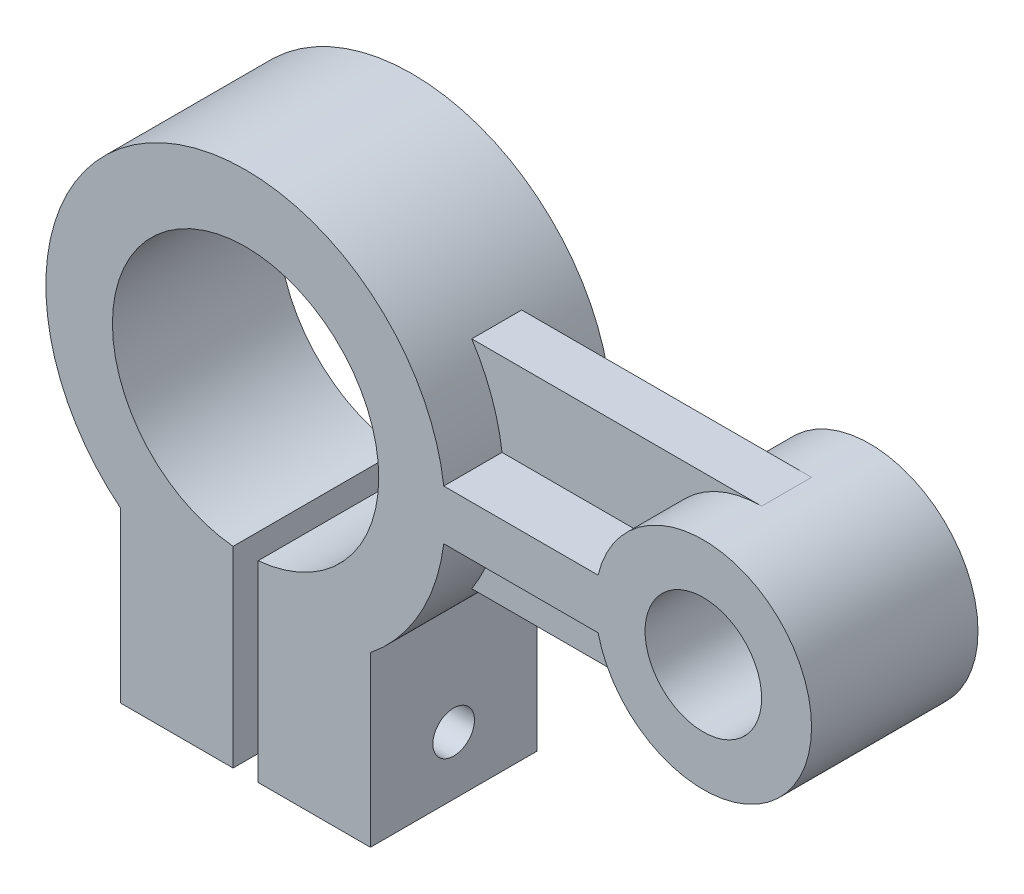
ISO-10303-21;
HEADER;
FILE_DESCRIPTION(('STEP AP214'),'2;1');
FILE_NAME('part.step','',(''),(''),'','','');
FILE_SCHEMA(('AUTOMOTIVE_DESIGN { 1 0 10303 214 1 1 1 1 }'));
ENDSEC;
DATA;
#1=APPLICATION_CONTEXT('core data for automotive mechanical design processes');
#2=APPLICATION_PROTOCOL_DEFINITION('international standard','automotive_design',2000,#1);
#3=PRODUCT_CONTEXT('',#1,'mechanical');
#4=PRODUCT('Part','Part','',(#3));
#5=PRODUCT_RELATED_PRODUCT_CATEGORY('part','',(#4));
#6=PRODUCT_DEFINITION_FORMATION('','',#4);
#7=PRODUCT_DEFINITION_CONTEXT('part definition',#1,'design');
#8=PRODUCT_DEFINITION('design','',#6,#7);
#9=PRODUCT_DEFINITION_SHAPE('','',#8);
#10=(LENGTH_UNIT() NAMED_UNIT(*) SI_UNIT(.MILLI.,.METRE.));
#11=(NAMED_UNIT(*) PLANE_ANGLE_UNIT() SI_UNIT($,.RADIAN.));
#12=(NAMED_UNIT(*) SI_UNIT($,.STERADIAN.) SOLID_ANGLE_UNIT());
#13=UNCERTAINTY_MEASURE_WITH_UNIT(LENGTH_MEASURE(1.E-05),#10,'distance_accuracy_value','');
#14=(GEOMETRIC_REPRESENTATION_CONTEXT(3) GLOBAL_UNCERTAINTY_ASSIGNED_CONTEXT((#13)) GLOBAL_UNIT_ASSIGNED_CONTEXT((#10,
#11,#12)) REPRESENTATION_CONTEXT('',''));
#15=CARTESIAN_POINT('',(0.,0.,0.));
#16=DIRECTION('',(0.,0.,1.));
#17=DIRECTION('',(1.,0.,0.));
#18=AXIS2_PLACEMENT_3D('',#15,#16,#17);
#19=CARTESIAN_POINT('',(47.6235235991626,72.,20.));
#20=DIRECTION('',(0.,1.,0.));
#21=DIRECTION('',(0.,0.,1.));
#22=AXIS2_PLACEMENT_3D('',#19,#20,#21);
#23=PLANE('',#22);
#24=DIRECTION('',(1.,0.,0.));
#25=VECTOR('',#24,1.);
#26=CARTESIAN_POINT('',(47.6235235991626,72.,-6.));
#27=LINE('',#26,#25);
#28=CARTESIAN_POINT('',(47.6235235991626,72.,-6.));
#29=VERTEX_POINT('',#28);
#30=CARTESIAN_POINT('',(84.7017787186529,72.,-6.));
#31=VERTEX_POINT('',#30);
#32=EDGE_CURVE('E193',#29,#31,#27,.T.);
#33=ORIENTED_EDGE('',*,*,#32,.F.);
#34=DIRECTION('',(0.,0.,-1.));
#35=VECTOR('',#34,1.);
#36=CARTESIAN_POINT('',(47.6235235991626,72.,20.));
#37=LINE('',#36,#35);
#38=CARTESIAN_POINT('',(47.6235235991626,72.,-20.));
#39=VERTEX_POINT('',#38);
#40=EDGE_CURVE('E277',#29,#39,#37,.T.);
#41=ORIENTED_EDGE('',*,*,#40,.T.);
#42=DIRECTION('',(1.,0.,0.));
#43=VECTOR('',#42,1.);
#44=CARTESIAN_POINT('',(47.6235235991626,72.,-20.));
#45=LINE('',#44,#43);
#46=CARTESIAN_POINT('',(84.7017787186529,72.,-20.));
#47=VERTEX_POINT('',#46);
#48=EDGE_CURVE('E250',#39,#47,#45,.T.);
#49=ORIENTED_EDGE('',*,*,#48,.T.);
#50=DIRECTION('',(0.,0.,-1.));
#51=VECTOR('',#50,1.);
#52=CARTESIAN_POINT('',(84.7017787186529,72.,20.));
#53=LINE('',#52,#51);
#54=EDGE_CURVE('E271',#31,#47,#53,.T.);
#55=ORIENTED_EDGE('',*,*,#54,.F.);
#56=EDGE_LOOP('',(#33,#41,#49,#55));
#57=FACE_BOUND('',#56,.T.);
#58=ADVANCED_FACE('F44',(#57),#23,.F.);
#59=CARTESIAN_POINT('',(47.6235235991626,84.,20.));
#60=DIRECTION('',(0.,-1.,0.));
#61=DIRECTION('',(0.,0.,-1.));
#62=AXIS2_PLACEMENT_3D('',#59,#60,#61);
#63=PLANE('',#62);
#64=DIRECTION('',(-1.,0.,0.));
#65=VECTOR('',#64,1.);
#66=CARTESIAN_POINT('',(47.6235235991626,84.,-6.));
#67=LINE('',#66,#65);
#68=CARTESIAN_POINT('',(84.7017787186529,84.,-6.));
#69=VERTEX_POINT('',#68);
#70=CARTESIAN_POINT('',(47.6235235991626,84.,-6.));
#71=VERTEX_POINT('',#70);
#72=EDGE_CURVE('E211',#69,#71,#67,.T.);
#73=ORIENTED_EDGE('',*,*,#72,.F.);
#74=DIRECTION('',(0.,0.,-1.));
#75=VECTOR('',#74,1.);
#76=CARTESIAN_POINT('',(84.7017787186529,84.,20.));
#77=LINE('',#76,#75);
#78=CARTESIAN_POINT('',(84.7017787186529,84.,-20.));
#79=VERTEX_POINT('',#78);
#80=EDGE_CURVE('E270',#69,#79,#77,.T.);
#81=ORIENTED_EDGE('',*,*,#80,.T.);
#82=DIRECTION('',(-1.,0.,0.));
#83=VECTOR('',#82,1.);
#84=CARTESIAN_POINT('',(47.6235235991626,84.,-20.));
#85=LINE('',#84,#83);
#86=CARTESIAN_POINT('',(47.6235235991626,84.,-20.));
#87=VERTEX_POINT('',#86);
#88=EDGE_CURVE('E254',#79,#87,#85,.T.);
#89=ORIENTED_EDGE('',*,*,#88,.T.);
#90=DIRECTION('',(0.,0.,-1.));
#91=VECTOR('',#90,1.);
#92=CARTESIAN_POINT('',(47.6235235991626,84.,20.));
#93=LINE('',#92,#91);
#94=EDGE_CURVE('E259',#71,#87,#93,.T.);
#95=ORIENTED_EDGE('',*,*,#94,.F.);
#96=EDGE_LOOP('',(#73,#81,#89,#95));
#97=FACE_BOUND('',#96,.T.);
#98=ADVANCED_FACE('F392',(#97),#63,.F.);
#99=CARTESIAN_POINT('',(0.,78.,20.));
#100=DIRECTION('',(0.,0.,-1.));
#101=DIRECTION('',(-1.,0.,0.));
#102=AXIS2_PLACEMENT_3D('',#99,#100,#101);
#103=CYLINDRICAL_SURFACE('',#102,48.);
#104=DIRECTION('',(0.,0.,-1.));
#105=VECTOR('',#104,1.);
#106=CARTESIAN_POINT('',(40.348482003664,52.,20.));
#107=LINE('',#106,#105);
#108=CARTESIAN_POINT('',(40.348482003664,52.,-6.));
#109=VERTEX_POINT('',#108);
#110=CARTESIAN_POINT('',(40.348482003664,52.,6.));
#111=VERTEX_POINT('',#110);
#112=EDGE_CURVE('E58',#109,#111,#107,.F.);
#113=ORIENTED_EDGE('',*,*,#112,.T.);
#114=CARTESIAN_POINT('',(0.,78.,6.));
#115=DIRECTION('',(0.,0.,1.));
#116=DIRECTION('',(1.,0.,0.));
#117=AXIS2_PLACEMENT_3D('',#114,#115,#116);
#118=CIRCLE('',#117,48.);
#119=CARTESIAN_POINT('',(47.6235235991626,72.,6.));
#120=VERTEX_POINT('',#119);
#121=EDGE_CURVE('E210',#111,#120,#118,.T.);
#122=ORIENTED_EDGE('',*,*,#121,.T.);
#123=CARTESIAN_POINT('',(47.6235235991626,72.,20.));
#124=VERTEX_POINT('',#123);
#125=EDGE_CURVE('E280',#124,#120,#37,.T.);
#126=ORIENTED_EDGE('',*,*,#125,.F.);
#127=CARTESIAN_POINT('',(0.,78.,20.));
#128=DIRECTION('',(0.,0.,1.));
#129=DIRECTION('',(1.,0.,0.));
#130=AXIS2_PLACEMENT_3D('',#127,#128,#129);
#131=CIRCLE('',#130,48.);
#132=CARTESIAN_POINT('',(30.,40.5300120096096,20.));
#133=VERTEX_POINT('',#132);
#134=EDGE_CURVE('E292',#133,#124,#131,.T.);
#135=ORIENTED_EDGE('',*,*,#134,.F.);
#136=DIRECTION('',(0.,0.,-1.));
#137=VECTOR('',#136,1.);
#138=CARTESIAN_POINT('',(30.,40.5300120096096,20.));
#139=LINE('',#138,#137);
#140=CARTESIAN_POINT('',(30.,40.5300120096096,-20.));
#141=VERTEX_POINT('',#140);
#142=EDGE_CURVE('E334',#133,#141,#139,.T.);
#143=ORIENTED_EDGE('',*,*,#142,.T.);
#144=CARTESIAN_POINT('',(0.,78.,-20.));
#145=DIRECTION('',(0.,0.,1.));
#146=DIRECTION('',(1.,0.,0.));
#147=AXIS2_PLACEMENT_3D('',#144,#145,#146);
#148=CIRCLE('',#147,48.);
#149=EDGE_CURVE('E313',#141,#39,#148,.T.);
#150=ORIENTED_EDGE('',*,*,#149,.T.);
#151=ORIENTED_EDGE('',*,*,#40,.F.);
#152=CARTESIAN_POINT('',(0.,78.,-6.));
#153=DIRECTION('',(0.,0.,1.));
#154=DIRECTION('',(1.,0.,0.));
#155=AXIS2_PLACEMENT_3D('',#152,#153,#154);
#156=CIRCLE('',#155,48.);
#157=EDGE_CURVE('E63',#109,#29,#156,.T.);
#158=ORIENTED_EDGE('',*,*,#157,.F.);
#159=EDGE_LOOP('',(#113,#122,#126,#135,#143,#150,#151,#158));
#160=FACE_BOUND('',#159,.T.);
#161=ADVANCED_FACE('F374',(#160),#103,.T.);
#162=CARTESIAN_POINT('',(0.,78.,6.));
#163=DIRECTION('',(0.,0.,1.));
#164=DIRECTION('',(1.,0.,0.));
#165=AXIS2_PLACEMENT_3D('',#162,#163,#164);
#166=CIRCLE('',#165,48.);
#167=CARTESIAN_POINT('',(47.6235235991626,84.,6.));
#168=VERTEX_POINT('',#167);
#169=CARTESIAN_POINT('',(40.348482003664,104.,6.));
#170=VERTEX_POINT('',#169);
#171=EDGE_CURVE('E230',#168,#170,#166,.T.);
#172=ORIENTED_EDGE('',*,*,#171,.T.);
#173=DIRECTION('',(0.,0.,-1.));
#174=VECTOR('',#173,1.);
#175=CARTESIAN_POINT('',(40.348482003664,104.,20.));
#176=LINE('',#175,#174);
#177=CARTESIAN_POINT('',(40.348482003664,104.,-6.));
#178=VERTEX_POINT('',#177);
#179=EDGE_CURVE('E233',#170,#178,#176,.T.);
#180=ORIENTED_EDGE('',*,*,#179,.T.);
#181=CARTESIAN_POINT('',(0.,78.,-6.));
#182=DIRECTION('',(0.,0.,1.));
#183=DIRECTION('',(1.,0.,0.));
#184=AXIS2_PLACEMENT_3D('',#181,#182,#183);
#185=CIRCLE('',#184,48.);
#186=EDGE_CURVE('E224',#71,#178,#185,.T.);
#187=ORIENTED_EDGE('',*,*,#186,.F.);
#188=ORIENTED_EDGE('',*,*,#94,.T.);
#189=CARTESIAN_POINT('',(-30.,40.5300120096096,-20.));
#190=VERTEX_POINT('',#189);
#191=EDGE_CURVE('E312',#87,#190,#148,.T.);
#192=ORIENTED_EDGE('',*,*,#191,.T.);
#193=DIRECTION('',(0.,0.,-1.));
#194=VECTOR('',#193,1.);
#195=CARTESIAN_POINT('',(-30.,40.5300120096096,20.));
#196=LINE('',#195,#194);
#197=CARTESIAN_POINT('',(-30.,40.5300120096096,20.));
#198=VERTEX_POINT('',#197);
#199=EDGE_CURVE('E328',#198,#190,#196,.T.);
#200=ORIENTED_EDGE('',*,*,#199,.F.);
#201=CARTESIAN_POINT('',(47.6235235991626,84.,20.));
#202=VERTEX_POINT('',#201);
#203=EDGE_CURVE('E293',#202,#198,#131,.T.);
#204=ORIENTED_EDGE('',*,*,#203,.F.);
#205=EDGE_CURVE('E268',#202,#168,#93,.T.);
#206=ORIENTED_EDGE('',*,*,#205,.T.);
#207=EDGE_LOOP('',(#172,#180,#187,#188,#192,#200,#204,#206));
#208=FACE_BOUND('',#207,.T.);
#209=ADVANCED_FACE('F354',(#208),#103,.T.);
#210=CARTESIAN_POINT('',(0.,78.,20.));
#211=DIRECTION('',(0.,0.,-1.));
#212=DIRECTION('',(-1.,0.,0.));
#213=AXIS2_PLACEMENT_3D('',#210,#211,#212);
#214=CYLINDRICAL_SURFACE('',#213,32.);
#215=CARTESIAN_POINT('',(0.,78.,-20.));
#216=DIRECTION('',(0.,0.,-1.));
#217=DIRECTION('',(1.,0.,0.));
#218=AXIS2_PLACEMENT_3D('',#215,#216,#217);
#219=CIRCLE('',#218,32.);
#220=CARTESIAN_POINT('',(-3.,46.140935355852,-20.));
#221=VERTEX_POINT('',#220);
#222=CARTESIAN_POINT('',(3.,46.140935355852,-20.));
#223=VERTEX_POINT('',#222);
#224=EDGE_CURVE('E278',#221,#223,#219,.T.);
#225=ORIENTED_EDGE('',*,*,#224,.T.);
#226=DIRECTION('',(0.,0.,-1.));
#227=VECTOR('',#226,1.);
#228=CARTESIAN_POINT('',(3.,46.140935355852,20.));
#229=LINE('',#228,#227);
#230=CARTESIAN_POINT('',(3.,46.140935355852,20.));
#231=VERTEX_POINT('',#230);
#232=EDGE_CURVE('E336',#231,#223,#229,.T.);
#233=ORIENTED_EDGE('',*,*,#232,.F.);
#234=CARTESIAN_POINT('',(0.,78.,20.));
#235=DIRECTION('',(0.,0.,-1.));
#236=DIRECTION('',(1.,0.,0.));
#237=AXIS2_PLACEMENT_3D('',#234,#235,#236);
#238=CIRCLE('',#237,32.);
#239=CARTESIAN_POINT('',(-3.,46.140935355852,20.));
#240=VERTEX_POINT('',#239);
#241=EDGE_CURVE('E282',#240,#231,#238,.T.);
#242=ORIENTED_EDGE('',*,*,#241,.F.);
#243=DIRECTION('',(0.,0.,-1.));
#244=VECTOR('',#243,1.);
#245=CARTESIAN_POINT('',(-3.,46.140935355852,20.));
#246=LINE('',#245,#244);
#247=EDGE_CURVE('E301',#240,#221,#246,.T.);
#248=ORIENTED_EDGE('',*,*,#247,.T.);
#249=EDGE_LOOP('',(#225,#233,#242,#248));
#250=FACE_BOUND('',#249,.T.);
#251=ADVANCED_FACE('F50',(#250),#214,.F.);
#252=CARTESIAN_POINT('',(3.,0.,20.));
#253=DIRECTION('',(1.,0.,0.));
#254=DIRECTION('',(0.,1.,0.));
#255=AXIS2_PLACEMENT_3D('',#252,#253,#254);
#256=PLANE('',#255);
#257=ORIENTED_EDGE('',*,*,#232,.T.);
#258=DIRECTION('',(0.,-1.,0.));
#259=VECTOR('',#258,1.);
#260=CARTESIAN_POINT('',(3.,0.,-20.));
#261=LINE('',#260,#259);
#262=CARTESIAN_POINT('',(3.,0.,-20.));
#263=VERTEX_POINT('',#262);
#264=EDGE_CURVE('E302',#223,#263,#261,.T.);
#265=ORIENTED_EDGE('',*,*,#264,.T.);
#266=DIRECTION('',(0.,0.,-1.));
#267=VECTOR('',#266,1.);
#268=CARTESIAN_POINT('',(3.,0.,20.));
#269=LINE('',#268,#267);
#270=CARTESIAN_POINT('',(3.,0.,20.));
#271=VERTEX_POINT('',#270);
#272=EDGE_CURVE('E337',#271,#263,#269,.T.);
#273=ORIENTED_EDGE('',*,*,#272,.F.);
#274=DIRECTION('',(0.,-1.,0.));
#275=VECTOR('',#274,1.);
#276=CARTESIAN_POINT('',(3.,0.,20.));
#277=LINE('',#276,#275);
#278=EDGE_CURVE('E281',#231,#271,#277,.T.);
#279=ORIENTED_EDGE('',*,*,#278,.F.);
#280=EDGE_LOOP('',(#257,#265,#273,#279));
#281=FACE_BOUND('',#280,.T.);
#282=CARTESIAN_POINT('',(3.00000000000001,14.,0.));
#283=DIRECTION('',(1.,0.,0.));
#284=DIRECTION('',(0.,1.,0.));
#285=AXIS2_PLACEMENT_3D('',#282,#283,#284);
#286=CIRCLE('',#285,5.);
#287=CARTESIAN_POINT('',(3.00000000000001,19.,0.));
#288=VERTEX_POINT('',#287);
#289=EDGE_CURVE('E239',#288,#288,#286,.T.);
#290=ORIENTED_EDGE('',*,*,#289,.T.);
#291=EDGE_LOOP('',(#290));
#292=FACE_BOUND('',#291,.T.);
#293=ADVANCED_FACE('F427',(#281,#292),#256,.F.);
#294=CARTESIAN_POINT('',(3.,0.,20.));
#295=DIRECTION('',(0.,1.,0.));
#296=DIRECTION('',(0.,0.,1.));
#297=AXIS2_PLACEMENT_3D('',#294,#295,#296);
#298=PLANE('',#297);
#299=ORIENTED_EDGE('',*,*,#272,.T.);
#300=DIRECTION('',(1.,0.,0.));
#301=VECTOR('',#300,1.);
#302=CARTESIAN_POINT('',(3.,0.,-20.));
#303=LINE('',#302,#301);
#304=CARTESIAN_POINT('',(30.,0.,-20.));
#305=VERTEX_POINT('',#304);
#306=EDGE_CURVE('E310',#263,#305,#303,.T.);
#307=ORIENTED_EDGE('',*,*,#306,.T.);
#308=DIRECTION('',(0.,0.,-1.));
#309=VECTOR('',#308,1.);
#310=CARTESIAN_POINT('',(30.,0.,20.));
#311=LINE('',#310,#309);
#312=CARTESIAN_POINT('',(30.,0.,20.));
#313=VERTEX_POINT('',#312);
#314=EDGE_CURVE('E335',#313,#305,#311,.T.);
#315=ORIENTED_EDGE('',*,*,#314,.F.);
#316=DIRECTION('',(1.,0.,0.));
#317=VECTOR('',#316,1.);
#318=CARTESIAN_POINT('',(3.,0.,20.));
#319=LINE('',#318,#317);
#320=EDGE_CURVE('E289',#271,#313,#319,.T.);
#321=ORIENTED_EDGE('',*,*,#320,.F.);
#322=EDGE_LOOP('',(#299,#307,#315,#321));
#323=FACE_BOUND('',#322,.T.);
#324=ADVANCED_FACE('F434',(#323),#298,.F.);
#325=CARTESIAN_POINT('',(30.,40.5300120096096,20.));
#326=DIRECTION('',(-1.,0.,0.));
#327=DIRECTION('',(0.,0.,1.));
#328=AXIS2_PLACEMENT_3D('',#325,#326,#327);
#329=PLANE('',#328);
#330=ORIENTED_EDGE('',*,*,#314,.T.);
#331=DIRECTION('',(0.,1.,0.));
#332=VECTOR('',#331,1.);
#333=CARTESIAN_POINT('',(30.,40.5300120096096,-20.));
#334=LINE('',#333,#332);
#335=EDGE_CURVE('E309',#305,#141,#334,.T.);
#336=ORIENTED_EDGE('',*,*,#335,.T.);
#337=ORIENTED_EDGE('',*,*,#142,.F.);
#338=DIRECTION('',(0.,1.,0.));
#339=VECTOR('',#338,1.);
#340=CARTESIAN_POINT('',(30.,40.5300120096096,20.));
#341=LINE('',#340,#339);
#342=EDGE_CURVE('E290',#313,#133,#341,.T.);
#343=ORIENTED_EDGE('',*,*,#342,.F.);
#344=EDGE_LOOP('',(#330,#336,#337,#343));
#345=FACE_BOUND('',#344,.T.);
#346=CARTESIAN_POINT('',(30.,14.,0.));
#347=DIRECTION('',(1.,0.,0.));
#348=DIRECTION('',(0.,0.,-1.));
#349=AXIS2_PLACEMENT_3D('',#346,#347,#348);
#350=CIRCLE('',#349,5.);
#351=CARTESIAN_POINT('',(30.,14.,-5.));
#352=VERTEX_POINT('',#351);
#353=EDGE_CURVE('E231',#352,#352,#350,.T.);
#354=ORIENTED_EDGE('',*,*,#353,.F.);
#355=EDGE_LOOP('',(#354));
#356=FACE_BOUND('',#355,.T.);
#357=ADVANCED_FACE('F438',(#345,#356),#329,.F.);
#358=CARTESIAN_POINT('',(-30.,40.5300120096096,20.));
#359=DIRECTION('',(1.,0.,0.));
#360=DIRECTION('',(0.,0.,-1.));
#361=AXIS2_PLACEMENT_3D('',#358,#359,#360);
#362=PLANE('',#361);
#363=ORIENTED_EDGE('',*,*,#199,.T.);
#364=DIRECTION('',(0.,-1.,0.));
#365=VECTOR('',#364,1.);
#366=CARTESIAN_POINT('',(-30.,40.5300120096096,-20.));
#367=LINE('',#366,#365);
#368=CARTESIAN_POINT('',(-30.,0.,-20.));
#369=VERTEX_POINT('',#368);
#370=EDGE_CURVE('E320',#190,#369,#367,.T.);
#371=ORIENTED_EDGE('',*,*,#370,.T.);
#372=DIRECTION('',(0.,0.,-1.));
#373=VECTOR('',#372,1.);
#374=CARTESIAN_POINT('',(-30.,0.,20.));
#375=LINE('',#374,#373);
#376=CARTESIAN_POINT('',(-30.,0.,20.));
#377=VERTEX_POINT('',#376);
#378=EDGE_CURVE('E329',#377,#369,#375,.T.);
#379=ORIENTED_EDGE('',*,*,#378,.F.);
#380=DIRECTION('',(0.,-1.,0.));
#381=VECTOR('',#380,1.);
#382=CARTESIAN_POINT('',(-30.,40.5300120096096,20.));
#383=LINE('',#382,#381);
#384=EDGE_CURVE('E294',#198,#377,#383,.T.);
#385=ORIENTED_EDGE('',*,*,#384,.F.);
#386=EDGE_LOOP('',(#363,#371,#379,#385));
#387=FACE_BOUND('',#386,.T.);
#388=CARTESIAN_POINT('',(-30.,14.,0.));
#389=DIRECTION('',(1.,0.,0.));
#390=DIRECTION('',(0.,0.,-1.));
#391=AXIS2_PLACEMENT_3D('',#388,#389,#390);
#392=CIRCLE('',#391,5.);
#393=CARTESIAN_POINT('',(-30.,14.,-5.));
#394=VERTEX_POINT('',#393);
#395=EDGE_CURVE('E234',#394,#394,#392,.T.);
#396=ORIENTED_EDGE('',*,*,#395,.T.);
#397=EDGE_LOOP('',(#396));
#398=FACE_BOUND('',#397,.T.);
#399=ADVANCED_FACE('F412',(#387,#398),#362,.F.);
#400=CARTESIAN_POINT('',(-30.,0.,20.));
#401=DIRECTION('',(0.,1.,0.));
#402=DIRECTION('',(0.,0.,1.));
#403=AXIS2_PLACEMENT_3D('',#400,#401,#402);
#404=PLANE('',#403);
#405=ORIENTED_EDGE('',*,*,#378,.T.);
#406=DIRECTION('',(1.,0.,0.));
#407=VECTOR('',#406,1.);
#408=CARTESIAN_POINT('',(-30.,0.,-20.));
#409=LINE('',#408,#407);
#410=CARTESIAN_POINT('',(-3.,0.,-20.));
#411=VERTEX_POINT('',#410);
#412=EDGE_CURVE('E318',#369,#411,#409,.T.);
#413=ORIENTED_EDGE('',*,*,#412,.T.);
#414=DIRECTION('',(0.,0.,-1.));
#415=VECTOR('',#414,1.);
#416=CARTESIAN_POINT('',(-3.,0.,20.));
#417=LINE('',#416,#415);
#418=CARTESIAN_POINT('',(-3.,0.,20.));
#419=VERTEX_POINT('',#418);
#420=EDGE_CURVE('E327',#419,#411,#417,.T.);
#421=ORIENTED_EDGE('',*,*,#420,.F.);
#422=DIRECTION('',(1.,0.,0.));
#423=VECTOR('',#422,1.);
#424=CARTESIAN_POINT('',(-30.,0.,20.));
#425=LINE('',#424,#423);
#426=EDGE_CURVE('E300',#377,#419,#425,.T.);
#427=ORIENTED_EDGE('',*,*,#426,.F.);
#428=EDGE_LOOP('',(#405,#413,#421,#427));
#429=FACE_BOUND('',#428,.T.);
#430=ADVANCED_FACE('F417',(#429),#404,.F.);
#431=CARTESIAN_POINT('',(-3.,0.,20.));
#432=DIRECTION('',(-1.,0.,0.));
#433=DIRECTION('',(0.,-1.,0.));
#434=AXIS2_PLACEMENT_3D('',#431,#432,#433);
#435=PLANE('',#434);
#436=ORIENTED_EDGE('',*,*,#420,.T.);
#437=DIRECTION('',(0.,1.,0.));
#438=VECTOR('',#437,1.);
#439=CARTESIAN_POINT('',(-3.,0.,-20.));
#440=LINE('',#439,#438);
#441=EDGE_CURVE('E283',#411,#221,#440,.T.);
#442=ORIENTED_EDGE('',*,*,#441,.T.);
#443=ORIENTED_EDGE('',*,*,#247,.F.);
#444=DIRECTION('',(0.,1.,0.));
#445=VECTOR('',#444,1.);
#446=CARTESIAN_POINT('',(-3.,0.,20.));
#447=LINE('',#446,#445);
#448=EDGE_CURVE('E299',#419,#240,#447,.T.);
#449=ORIENTED_EDGE('',*,*,#448,.F.);
#450=EDGE_LOOP('',(#436,#442,#443,#449));
#451=FACE_BOUND('',#450,.T.);
#452=CARTESIAN_POINT('',(-3.,14.,0.));
#453=DIRECTION('',(-1.,0.,0.));
#454=DIRECTION('',(0.,-1.,0.));
#455=AXIS2_PLACEMENT_3D('',#452,#453,#454);
#456=CIRCLE('',#455,5.);
#457=CARTESIAN_POINT('',(-3.,9.,0.));
#458=VERTEX_POINT('',#457);
#459=EDGE_CURVE('E240',#458,#458,#456,.T.);
#460=ORIENTED_EDGE('',*,*,#459,.T.);
#461=EDGE_LOOP('',(#460));
#462=FACE_BOUND('',#461,.T.);
#463=ADVANCED_FACE('F423',(#451,#462),#435,.F.);
#464=CARTESIAN_POINT('',(0.,78.,20.));
#465=DIRECTION('',(0.,0.,1.));
#466=DIRECTION('',(1.,0.,0.));
#467=AXIS2_PLACEMENT_3D('',#464,#465,#466);
#468=PLANE('',#467);
#469=ORIENTED_EDGE('',*,*,#241,.T.);
#470=ORIENTED_EDGE('',*,*,#278,.T.);
#471=ORIENTED_EDGE('',*,*,#320,.T.);
#472=ORIENTED_EDGE('',*,*,#342,.T.);
#473=ORIENTED_EDGE('',*,*,#134,.T.);
#474=DIRECTION('',(1.,0.,0.));
#475=VECTOR('',#474,1.);
#476=CARTESIAN_POINT('',(47.6235235991626,72.,20.));
#477=LINE('',#476,#475);
#478=CARTESIAN_POINT('',(84.7017787186529,72.,20.));
#479=VERTEX_POINT('',#478);
#480=EDGE_CURVE('E249',#124,#479,#477,.T.);
#481=ORIENTED_EDGE('',*,*,#480,.T.);
#482=CARTESIAN_POINT('',(110.,78.,20.));
#483=DIRECTION('',(0.,0.,1.));
#484=DIRECTION('',(1.,0.,0.));
#485=AXIS2_PLACEMENT_3D('',#482,#483,#484);
#486=CIRCLE('',#485,26.);
#487=CARTESIAN_POINT('',(84.7017787186529,84.,20.));
#488=VERTEX_POINT('',#487);
#489=EDGE_CURVE('E255',#479,#488,#486,.T.);
#490=ORIENTED_EDGE('',*,*,#489,.T.);
#491=DIRECTION('',(-1.,0.,0.));
#492=VECTOR('',#491,1.);
#493=CARTESIAN_POINT('',(47.6235235991626,84.,20.));
#494=LINE('',#493,#492);
#495=EDGE_CURVE('E253',#488,#202,#494,.T.);
#496=ORIENTED_EDGE('',*,*,#495,.T.);
#497=ORIENTED_EDGE('',*,*,#203,.T.);
#498=ORIENTED_EDGE('',*,*,#384,.T.);
#499=ORIENTED_EDGE('',*,*,#426,.T.);
#500=ORIENTED_EDGE('',*,*,#448,.T.);
#501=EDGE_LOOP('',(#469,#470,#471,#472,#473,#481,#490,#496,#497,#498,#499,#500));
#502=FACE_BOUND('',#501,.T.);
#503=CARTESIAN_POINT('',(110.,78.,20.));
#504=DIRECTION('',(0.,0.,1.));
#505=DIRECTION('',(1.,0.,0.));
#506=AXIS2_PLACEMENT_3D('',#503,#504,#505);
#507=CIRCLE('',#506,14.);
#508=CARTESIAN_POINT('',(124.,78.,20.));
#509=VERTEX_POINT('',#508);
#510=EDGE_CURVE('E242',#509,#509,#507,.T.);
#511=ORIENTED_EDGE('',*,*,#510,.F.);
#512=EDGE_LOOP('',(#511));
#513=FACE_BOUND('',#512,.T.);
#514=ADVANCED_FACE('F366',(#502,#513),#468,.T.);
#515=CARTESIAN_POINT('',(0.,78.,-20.));
#516=DIRECTION('',(0.,0.,1.));
#517=DIRECTION('',(1.,0.,0.));
#518=AXIS2_PLACEMENT_3D('',#515,#516,#517);
#519=PLANE('',#518);
#520=ORIENTED_EDGE('',*,*,#224,.F.);
#521=ORIENTED_EDGE('',*,*,#441,.F.);
#522=ORIENTED_EDGE('',*,*,#412,.F.);
#523=ORIENTED_EDGE('',*,*,#370,.F.);
#524=ORIENTED_EDGE('',*,*,#191,.F.);
#525=ORIENTED_EDGE('',*,*,#88,.F.);
#526=CARTESIAN_POINT('',(110.,78.,-20.));
#527=DIRECTION('',(0.,0.,1.));
#528=DIRECTION('',(1.,0.,0.));
#529=AXIS2_PLACEMENT_3D('',#526,#527,#528);
#530=CIRCLE('',#529,26.);
#531=EDGE_CURVE('E262',#47,#79,#530,.T.);
#532=ORIENTED_EDGE('',*,*,#531,.F.);
#533=ORIENTED_EDGE('',*,*,#48,.F.);
#534=ORIENTED_EDGE('',*,*,#149,.F.);
#535=ORIENTED_EDGE('',*,*,#335,.F.);
#536=ORIENTED_EDGE('',*,*,#306,.F.);
#537=ORIENTED_EDGE('',*,*,#264,.F.);
#538=EDGE_LOOP('',(#520,#521,#522,#523,#524,#525,#532,#533,#534,#535,#536,#537));
#539=FACE_BOUND('',#538,.T.);
#540=CARTESIAN_POINT('',(110.,78.,-20.));
#541=DIRECTION('',(0.,0.,1.));
#542=DIRECTION('',(1.,0.,0.));
#543=AXIS2_PLACEMENT_3D('',#540,#541,#542);
#544=CIRCLE('',#543,14.);
#545=CARTESIAN_POINT('',(124.,78.,-20.));
#546=VERTEX_POINT('',#545);
#547=EDGE_CURVE('E243',#546,#546,#544,.T.);
#548=ORIENTED_EDGE('',*,*,#547,.T.);
#549=EDGE_LOOP('',(#548));
#550=FACE_BOUND('',#549,.T.);
#551=ADVANCED_FACE('F378',(#539,#550),#519,.F.);
#552=ORIENTED_EDGE('',*,*,#125,.T.);
#553=DIRECTION('',(1.,0.,0.));
#554=VECTOR('',#553,1.);
#555=CARTESIAN_POINT('',(47.6235235991626,72.,6.));
#556=LINE('',#555,#554);
#557=CARTESIAN_POINT('',(84.7017787186529,72.,6.));
#558=VERTEX_POINT('',#557);
#559=EDGE_CURVE('E201',#120,#558,#556,.T.);
#560=ORIENTED_EDGE('',*,*,#559,.T.);
#561=EDGE_CURVE('E274',#479,#558,#53,.T.);
#562=ORIENTED_EDGE('',*,*,#561,.F.);
#563=ORIENTED_EDGE('',*,*,#480,.F.);
#564=EDGE_LOOP('',(#552,#560,#562,#563));
#565=FACE_BOUND('',#564,.T.);
#566=ADVANCED_FACE('F380',(#565),#23,.F.);
#567=CARTESIAN_POINT('',(110.,78.,20.));
#568=DIRECTION('',(0.,0.,-1.));
#569=DIRECTION('',(-1.,0.,0.));
#570=AXIS2_PLACEMENT_3D('',#567,#568,#569);
#571=CYLINDRICAL_SURFACE('',#570,26.);
#572=CARTESIAN_POINT('',(110.,78.,6.));
#573=DIRECTION('',(0.,0.,1.));
#574=DIRECTION('',(1.,0.,0.));
#575=AXIS2_PLACEMENT_3D('',#572,#573,#574);
#576=CIRCLE('',#575,26.);
#577=CARTESIAN_POINT('',(110.,52.,6.));
#578=VERTEX_POINT('',#577);
#579=EDGE_CURVE('E184',#558,#578,#576,.T.);
#580=ORIENTED_EDGE('',*,*,#579,.T.);
#581=DIRECTION('',(0.,0.,-1.));
#582=VECTOR('',#581,1.);
#583=CARTESIAN_POINT('',(110.,52.,20.));
#584=LINE('',#583,#582);
#585=CARTESIAN_POINT('',(110.,52.,-6.));
#586=VERTEX_POINT('',#585);
#587=EDGE_CURVE('E11',#586,#578,#584,.F.);
#588=ORIENTED_EDGE('',*,*,#587,.F.);
#589=CARTESIAN_POINT('',(110.,78.,-6.));
#590=DIRECTION('',(0.,0.,1.));
#591=DIRECTION('',(1.,0.,0.));
#592=AXIS2_PLACEMENT_3D('',#589,#590,#591);
#593=CIRCLE('',#592,26.);
#594=EDGE_CURVE('E181',#31,#586,#593,.T.);
#595=ORIENTED_EDGE('',*,*,#594,.F.);
#596=ORIENTED_EDGE('',*,*,#54,.T.);
#597=ORIENTED_EDGE('',*,*,#531,.T.);
#598=ORIENTED_EDGE('',*,*,#80,.F.);
#599=CARTESIAN_POINT('',(110.,78.,-6.));
#600=DIRECTION('',(0.,0.,1.));
#601=DIRECTION('',(1.,0.,0.));
#602=AXIS2_PLACEMENT_3D('',#599,#600,#601);
#603=CIRCLE('',#602,26.);
#604=CARTESIAN_POINT('',(110.,104.,-6.));
#605=VERTEX_POINT('',#604);
#606=EDGE_CURVE('E216',#605,#69,#603,.T.);
#607=ORIENTED_EDGE('',*,*,#606,.F.);
#608=DIRECTION('',(0.,0.,-1.));
#609=VECTOR('',#608,1.);
#610=CARTESIAN_POINT('',(110.,104.,20.));
#611=LINE('',#610,#609);
#612=CARTESIAN_POINT('',(110.,104.,6.));
#613=VERTEX_POINT('',#612);
#614=EDGE_CURVE('E52',#613,#605,#611,.T.);
#615=ORIENTED_EDGE('',*,*,#614,.F.);
#616=CARTESIAN_POINT('',(110.,78.,6.));
#617=DIRECTION('',(0.,0.,1.));
#618=DIRECTION('',(1.,0.,0.));
#619=AXIS2_PLACEMENT_3D('',#616,#617,#618);
#620=CIRCLE('',#619,26.);
#621=CARTESIAN_POINT('',(84.7017787186529,84.,6.));
#622=VERTEX_POINT('',#621);
#623=EDGE_CURVE('E227',#613,#622,#620,.T.);
#624=ORIENTED_EDGE('',*,*,#623,.T.);
#625=EDGE_CURVE('E266',#488,#622,#77,.T.);
#626=ORIENTED_EDGE('',*,*,#625,.F.);
#627=ORIENTED_EDGE('',*,*,#489,.F.);
#628=ORIENTED_EDGE('',*,*,#561,.T.);
#629=EDGE_LOOP('',(#580,#588,#595,#596,#597,#598,#607,#615,#624,#626,#627,#628));
#630=FACE_BOUND('',#629,.T.);
#631=ADVANCED_FACE('F179',(#630),#571,.T.);
#632=ORIENTED_EDGE('',*,*,#625,.T.);
#633=DIRECTION('',(-1.,0.,0.));
#634=VECTOR('',#633,1.);
#635=CARTESIAN_POINT('',(47.6235235991626,84.,6.));
#636=LINE('',#635,#634);
#637=EDGE_CURVE('E221',#622,#168,#636,.T.);
#638=ORIENTED_EDGE('',*,*,#637,.T.);
#639=ORIENTED_EDGE('',*,*,#205,.F.);
#640=ORIENTED_EDGE('',*,*,#495,.F.);
#641=EDGE_LOOP('',(#632,#638,#639,#640));
#642=FACE_BOUND('',#641,.T.);
#643=ADVANCED_FACE('F361',(#642),#63,.F.);
#644=CARTESIAN_POINT('',(110.,78.,20.));
#645=DIRECTION('',(0.,0.,-1.));
#646=DIRECTION('',(-1.,0.,0.));
#647=AXIS2_PLACEMENT_3D('',#644,#645,#646);
#648=CYLINDRICAL_SURFACE('',#647,14.);
#649=ORIENTED_EDGE('',*,*,#510,.T.);
#650=EDGE_LOOP('',(#649));
#651=FACE_BOUND('',#650,.T.);
#652=ORIENTED_EDGE('',*,*,#547,.F.);
#653=EDGE_LOOP('',(#652));
#654=FACE_BOUND('',#653,.T.);
#655=ADVANCED_FACE('F483',(#651,#654),#648,.F.);
#656=CARTESIAN_POINT('',(-30.,14.,0.));
#657=DIRECTION('',(1.,0.,0.));
#658=DIRECTION('',(0.,0.,-1.));
#659=AXIS2_PLACEMENT_3D('',#656,#657,#658);
#660=CYLINDRICAL_SURFACE('',#659,5.);
#661=ORIENTED_EDGE('',*,*,#395,.F.);
#662=EDGE_LOOP('',(#661));
#663=FACE_BOUND('',#662,.T.);
#664=ORIENTED_EDGE('',*,*,#459,.F.);
#665=EDGE_LOOP('',(#664));
#666=FACE_BOUND('',#665,.T.);
#667=ADVANCED_FACE('F450',(#663,#666),#660,.F.);
#668=ORIENTED_EDGE('',*,*,#353,.T.);
#669=EDGE_LOOP('',(#668));
#670=FACE_BOUND('',#669,.T.);
#671=ORIENTED_EDGE('',*,*,#289,.F.);
#672=EDGE_LOOP('',(#671));
#673=FACE_BOUND('',#672,.T.);
#674=ADVANCED_FACE('F443',(#670,#673),#660,.F.);
#675=CARTESIAN_POINT('',(110.,104.,0.));
#676=DIRECTION('',(0.,1.,0.));
#677=DIRECTION('',(-1.,0.,0.));
#678=AXIS2_PLACEMENT_3D('',#675,#676,#677);
#679=PLANE('',#678);
#680=ORIENTED_EDGE('',*,*,#179,.F.);
#681=DIRECTION('',(1.,0.,0.));
#682=VECTOR('',#681,1.);
#683=CARTESIAN_POINT('',(44.,104.,6.));
#684=LINE('',#683,#682);
#685=EDGE_CURVE('E212',#613,#170,#684,.F.);
#686=ORIENTED_EDGE('',*,*,#685,.F.);
#687=ORIENTED_EDGE('',*,*,#614,.T.);
#688=DIRECTION('',(1.,0.,0.));
#689=VECTOR('',#688,1.);
#690=CARTESIAN_POINT('',(44.,104.,-6.));
#691=LINE('',#690,#689);
#692=EDGE_CURVE('E208',#605,#178,#691,.F.);
#693=ORIENTED_EDGE('',*,*,#692,.T.);
#694=EDGE_LOOP('',(#680,#686,#687,#693));
#695=FACE_BOUND('',#694,.T.);
#696=ADVANCED_FACE('F347',(#695),#679,.T.);
#697=CARTESIAN_POINT('',(44.,63.,6.));
#698=DIRECTION('',(0.,0.,1.));
#699=DIRECTION('',(1.,0.,0.));
#700=AXIS2_PLACEMENT_3D('',#697,#698,#699);
#701=PLANE('',#700);
#702=ORIENTED_EDGE('',*,*,#171,.F.);
#703=ORIENTED_EDGE('',*,*,#637,.F.);
#704=ORIENTED_EDGE('',*,*,#623,.F.);
#705=ORIENTED_EDGE('',*,*,#685,.T.);
#706=EDGE_LOOP('',(#702,#703,#704,#705));
#707=FACE_BOUND('',#706,.T.);
#708=ADVANCED_FACE('F357',(#707),#701,.T.);
#709=CARTESIAN_POINT('',(44.,63.,-6.));
#710=DIRECTION('',(0.,0.,1.));
#711=DIRECTION('',(1.,0.,0.));
#712=AXIS2_PLACEMENT_3D('',#709,#710,#711);
#713=PLANE('',#712);
#714=ORIENTED_EDGE('',*,*,#72,.T.);
#715=ORIENTED_EDGE('',*,*,#186,.T.);
#716=ORIENTED_EDGE('',*,*,#692,.F.);
#717=ORIENTED_EDGE('',*,*,#606,.T.);
#718=EDGE_LOOP('',(#714,#715,#716,#717));
#719=FACE_BOUND('',#718,.T.);
#720=ADVANCED_FACE('F346',(#719),#713,.F.);
#721=CARTESIAN_POINT('',(110.,52.,0.));
#722=DIRECTION('',(0.,1.,0.));
#723=DIRECTION('',(-1.,0.,0.));
#724=AXIS2_PLACEMENT_3D('',#721,#722,#723);
#725=PLANE('',#724);
#726=ORIENTED_EDGE('',*,*,#112,.F.);
#727=DIRECTION('',(1.,0.,0.));
#728=VECTOR('',#727,1.);
#729=CARTESIAN_POINT('',(44.,52.,-6.));
#730=LINE('',#729,#728);
#731=EDGE_CURVE('E191',#586,#109,#730,.F.);
#732=ORIENTED_EDGE('',*,*,#731,.F.);
#733=ORIENTED_EDGE('',*,*,#587,.T.);
#734=DIRECTION('',(1.,0.,0.));
#735=VECTOR('',#734,1.);
#736=CARTESIAN_POINT('',(44.,52.,6.));
#737=LINE('',#736,#735);
#738=EDGE_CURVE('E197',#578,#111,#737,.F.);
#739=ORIENTED_EDGE('',*,*,#738,.T.);
#740=EDGE_LOOP('',(#726,#732,#733,#739));
#741=FACE_BOUND('',#740,.T.);
#742=ADVANCED_FACE('F199',(#741),#725,.F.);
#743=CARTESIAN_POINT('',(44.,63.,6.));
#744=DIRECTION('',(0.,0.,1.));
#745=DIRECTION('',(1.,0.,0.));
#746=AXIS2_PLACEMENT_3D('',#743,#744,#745);
#747=PLANE('',#746);
#748=ORIENTED_EDGE('',*,*,#121,.F.);
#749=ORIENTED_EDGE('',*,*,#738,.F.);
#750=ORIENTED_EDGE('',*,*,#579,.F.);
#751=ORIENTED_EDGE('',*,*,#559,.F.);
#752=EDGE_LOOP('',(#748,#749,#750,#751));
#753=FACE_BOUND('',#752,.T.);
#754=ADVANCED_FACE('F372',(#753),#747,.T.);
#755=CARTESIAN_POINT('',(44.,63.,-6.));
#756=DIRECTION('',(0.,0.,1.));
#757=DIRECTION('',(1.,0.,0.));
#758=AXIS2_PLACEMENT_3D('',#755,#756,#757);
#759=PLANE('',#758);
#760=ORIENTED_EDGE('',*,*,#731,.T.);
#761=ORIENTED_EDGE('',*,*,#157,.T.);
#762=ORIENTED_EDGE('',*,*,#32,.T.);
#763=ORIENTED_EDGE('',*,*,#594,.T.);
#764=EDGE_LOOP('',(#760,#761,#762,#763));
#765=FACE_BOUND('',#764,.T.);
#766=ADVANCED_FACE('F194',(#765),#759,.F.);
#767=CLOSED_SHELL('',(#58,#98,#161,#209,#251,#293,#324,#357,#399,#430,#463,#514,#551,#566,#631,
#643,#655,#667,#674,#696,#708,#720,#742,#754,#766));
#768=MANIFOLD_SOLID_BREP('B2',#767);
#769=ADVANCED_BREP_SHAPE_REPRESENTATION('',(#18,#768),#14);
#770=SHAPE_DEFINITION_REPRESENTATION(#9,#769);
ENDSEC;
END-ISO-10303-21;
